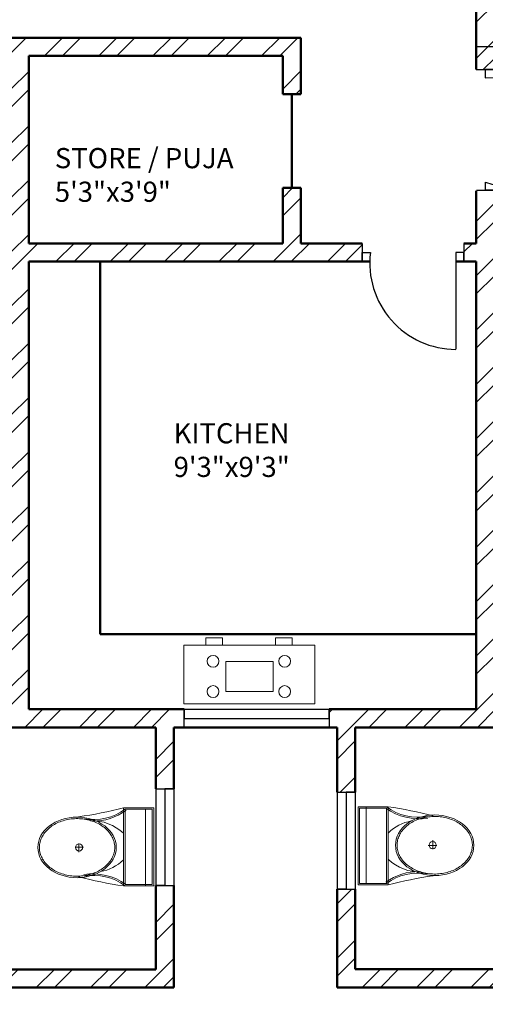
# Model space of a CAD drawing. Units: inches. Extents: x 963 to 2075, y 289 to 2657.
# Tile 4 of 98: x 1259 to 1374, y 1474 to 1718. Entities that reach past the tile are written whole.
import ezdxf

# ---------------------------------------------------------------- set-up
doc = ezdxf.new("R2010")
doc.units = ezdxf.units.IN
for name, color, linetype, lineweight in [('A-ANNO-DIMS', 2, 'Continuous', 18), ('A-AREA-IDEN', 7, 'Continuous', 18), ('A-DOOR', 4, 'Continuous', 25), ('A-FLOR-FIXT', 9, 'Continuous', 18), ('A-GLAZ', 3, 'Continuous', 25), ('A-WALL', 7, 'Continuous', 50), ('A-WALL-PATT', 8, 'Continuous', 13)]:
    doc.layers.add(name, color=color, linetype=linetype, lineweight=lineweight)
doc.styles.get("Standard").update_dxf_attribs({"font": 'arial.ttf'})
doc.dimstyles.get("Standard").update_dxf_attribs({"dimtxt": 0.18, "dimasz": 0.18, "dimexe": 0.18, "dimexo": 0.0625, "dimgap": 0.09, "dimtad": 0, "dimtih": 1, "dimtoh": 1, "dimdec": 4, "dimzin": 0, "dimdsep": 46, "dimtxsty": 'Standard', "dimcen": 0.09, "dimadec": 0, "dimazin": 0, "dimtfac": 1, "dimtdec": 4, "dimtofl": 0, "dimtmove": 0, "dimatfit": 3, "dimfxl": 1, "dimtolj": 1, "dimtzin": 0, "dimarcsym": 0})

# ---------------------------------------------------------------- blocks, each defined once
blk = doc.blocks.new('A$C31115884')
for p, q in [((283.1, 497.7), (223.4, 497.7)), ((257.5, 466.4), (257.5, 523.2)), ((0, 200), (0, 0)), ((520, 200), (0, 200)), ((520, 0), (520, 200)), ((10, 190), (10, 10)), ((510, 190), (10, 190)), ((510, 10), (510, 190)), ((510, 54.5), (0, 54.5)), ((10, 10), (510, 10)), ((0, 0), (520, 0))]:
    blk.add_line(p, q)
blk.add_circle((255.6, 496.4), 23.6)
for centre, radius, start, end in [((2777.7, -204.6), 2807, 165.4549, 171.71327), ((-294.5, 403.3), 364.7, 324.20913, 9.34987), ((-294.5, 403.3), 374.7, 324.20913, 9.34987), ((805.8, 403.3), 364.7, 170.65013, 215.79087), ((3237, 905), 2807, 188.28673, 194.5451), ((139.5, 406.2), 293.5, 315.84364, 2.65635), ((805.8, 403.3), 374.7, 179.20365, 215.79087), ((383.6, 406.2), 293.5, 190.27735, 224.15636)]:
    blk.add_arc(centre, radius, start, end)
blk.add_ellipse((256.2, 509.9), major_axis=(0, -260.7), ratio=0.772727)
blk.add_open_spline([(256.2, 259.2), (263.1, 259.2), (270, 259.7), (287.8, 262.3), (298.7, 265.1), (319.9, 273.1), (330.2, 278.4), (350.1, 291.1), (359.7, 298.7), (377.7, 315.9), (386.2, 325.5), (401.7, 346.6), (408.8, 358.1), (421.3, 382.5), (426.8, 395.5), (435.9, 422.4), (439.5, 436.4), (444.8, 465.1), (446.5, 479.7), (447.9, 509.2), (447.6, 524), (445, 553.3), (442.7, 567.8), (436.3, 596), (432.1, 609.7), (421.9, 636), (416, 648.6), (402.5, 672.1), (395, 683), (378.6, 703), (369.8, 712.1), (351.1, 728), (341.3, 734.8), (320.9, 746.2), (310.4, 750.7), (288.9, 757.3), (278, 759.4), (256, 761), (245, 760.6), (223.1, 757.2), (212.3, 754.3), (191.1, 746.1), (180.8, 740.7), (160.9, 727.8), (151.4, 720.1), (133.5, 702.7), (125.1, 693), (109.6, 671.7), (102.6, 660.2), (90.2, 635.7), (84.9, 622.7), (76, 595.6), (72.4, 581.6), (67.2, 552.9), (65.6, 538.2), (64.4, 508.8), (64.8, 494), (67.5, 464.7), (69.9, 450.2), (76.6, 422), (80.8, 408.3), (91.1, 382.2), (97.2, 369.7), (110.8, 346.3), (118.4, 335.4), (134.8, 315.6), (143.7, 306.7), (162.4, 290.9), (172.3, 284.2), (192.8, 273), (203.3, 268.6), (224.8, 262.2), (235.8, 260.2), (249.9, 259.3), (253, 259.2), (256.2, 259.2)], degree=3, knots=[0, 0, 0, 0, 0.110105, 0.110105, 0.285049, 0.285049, 0.459994, 0.459994, 0.634938, 0.634938, 0.809882, 0.809882, 0.984827, 0.984827, 1.159771, 1.159771, 1.334715, 1.334715, 1.50966, 1.50966, 1.684604, 1.684604, 1.859549, 1.859549, 2.034493, 2.034493, 2.209437, 2.209437, 2.384382, 2.384382, 2.559326, 2.559326, 2.73427, 2.73427, 2.909215, 2.909215, 3.084159, 3.084159, 3.259103, 3.259103, 3.434048, 3.434048, 3.608992, 3.608992, 3.783936, 3.783936, 3.958881, 3.958881, 4.133825, 4.133825, 4.30877, 4.30877, 4.483714, 4.483714, 4.658658, 4.658658, 4.833603, 4.833603, 5.008547, 5.008547, 5.183491, 5.183491, 5.358436, 5.358436, 5.53338, 5.53338, 5.708324, 5.708324, 5.883269, 5.883269, 6.058213, 6.058213, 6.233158, 6.233158, 6.283185, 6.283185, 6.283185, 6.283185])
blk = doc.blocks.new('DOOR-5')
for p, q in [((0, 38.25), (0, 33.75)), ((29.91, 38.25), (29.91, 33.75)), ((0, 33.75), (0, 36)), ((0, 36), (2, 36)), ((29.91, 36), (27.91, 36)), ((27.91, 36), (27.91, 0)), ((29.91, 33.75), (29.91, 36))]:
    blk.add_line(p, q)
blk.add_arc((27.91, 27.32), 27.32, 161.4794, 270)
blk = doc.blocks.new('*D38')
at = {"layer": 'A-ANNO-DIMS', "color": 0, "lineweight": -2, "transparency": 16777216}
for p, q in [((1371.88, 1705.97), (1371.87, 1711.82)), ((1372.05, 1711.64), (1389.86, 1711.69)), ((1409.94, 1711.73), (1392.12, 1711.69)), ((1410.13, 1706.06), (1410.12, 1711.92))]:
    blk.add_line(p, q, dxfattribs=at)
at = {"layer": 'A-ANNO-DIMS', "color": 0, "transparency": 16777216}
for points in [[(1372.05, 1711.67), (1372.05, 1711.61), (1371.87, 1711.64)], [(1409.94, 1711.76), (1409.94, 1711.7), (1410.12, 1711.74)]]:
    blk.add_solid(points, dxfattribs=at)
at = {"layer": 'Defpoints', "color": 0, "transparency": 16777216}
for p in [(1371.87, 1711.64), (1371.88, 1705.9), (1410.13, 1706)]:
    blk.add_point(p, dxfattribs=at)
at = {"layer": 'A-ANNO-DIMS', "color": 0, "transparency": 16777216, "insert": (1390.99, 1711.69), "char_height": 0.18, "attachment_point": 5}
blk.add_mtext('\\A1;DOOR D5 38 TYP.', dxfattribs=at)

msp = doc.modelspace()

# ---------------------------------------------------------------- hatches: boundary and pattern name
at = {"layer": 'A-WALL-PATT'}
h = msp.add_hatch(dxfattribs=at)
h.set_pattern_fill('ANSI32', color=256)
h.paths.add_polyline_path([(1296.92, 2558.32), (1203.92, 2558.32), (1203.92, 2493.82), (1191.53, 2493.82), (1191.53, 2489.32), (1211.06, 2489.32), (1211.06, 2492.02), (1211.06, 2493.82), (1208.42, 2493.82), (1208.42, 2553.82), (1292.42, 2553.82), (1292.42, 2538.86), (1296.92, 2538.86)])
h.paths.add_polyline_path([(1442.42, 2558.32), (1349.42, 2558.32), (1349.42, 2538.94), (1353.92, 2538.94), (1353.92, 2553.82), (1437.92, 2553.82), (1437.92, 2493.82), (1434.54, 2493.82), (1434.54, 2489.32), (1448.31, 2489.32), (1448.31, 2491.57), (1448.31, 2493.82), (1442.42, 2493.82)])
h.paths.add_polyline_path([(1415.55, 2491.57), (1415.55, 2493.82), (1340.94, 2493.82), (1340.94, 2489.32), (1371.92, 2489.32), (1371.92, 2378.32), (1367.6, 2378.32), (1367.6, 2373.82), (1371.92, 2373.82), (1371.92, 2355.19), (1376.42, 2355.19), (1376.42, 2489.32), (1415.55, 2489.32)])
h.paths.add_polyline_path([(1304.94, 2491.57), (1304.94, 2493.82), (1296.92, 2493.82), (1296.92, 2514.86), (1292.42, 2514.86), (1292.42, 2493.82), (1232.81, 2493.82), (1232.81, 2489.32), (1256.42, 2489.32), (1256.42, 2327.32), (1253.71, 2327.32), (1253.71, 2322.82), (1328.42, 2322.82), (1328.42, 2331.15), (1323.92, 2331.15), (1323.92, 2327.32), (1260.92, 2327.32), (1260.92, 2373.82), (1323.92, 2373.82), (1323.92, 2357.81), (1328.42, 2357.81), (1328.42, 2373.82), (1346.01, 2373.82), (1346.01, 2376.07), (1346.01, 2378.32), (1260.92, 2378.32), (1260.92, 2489.32), (1304.94, 2489.32)])
h.paths.add_polyline_path([(1226.65, 2327.32), (1124.42, 2327.32), (1124.42, 2347.45), (1119.92, 2347.45), (1119.92, 2322.82), (1163.42, 2322.82), (1163.42, 2305.43), (1165.67, 2305.43), (1167.92, 2305.43), (1167.92, 2322.82), (1226.65, 2322.82), (1226.65, 2325.07)])
h.paths.add_polyline_path([(1095.92, 2489.32), (1124.42, 2489.32), (1131.53, 2489.32), (1131.53, 2491.57), (1131.53, 2493.82), (1119.92, 2493.82), (1091.42, 2493.82), (1091.42, 2417.32), (1095.92, 2417.32), (1119.92, 2417.32), (1119.92, 2407.45), (1124.42, 2407.45), (1124.42, 2421.82), (1095.92, 2421.82)])
h.paths.add_polyline_path([(1512.92, 2558.32), (1508.42, 2558.32), (1508.42, 2493.82), (1503.4, 2493.82), (1503.4, 2489.32), (1508.42, 2489.32), (1508.42, 2327.32), (1376.42, 2327.32), (1376.42, 2330.27), (1371.92, 2330.27), (1371.92, 2298.74), (1376.42, 2298.74), (1376.42, 2322.82), (1508.42, 2322.82), (1508.42, 2165.32), (1504.26, 2165.32), (1504.26, 2160.82), (1508.42, 2160.82), (1508.42, 2108.32), (1512.92, 2108.32), (1512.92, 2160.82), (1516.18, 2160.82), (1516.18, 2163.07), (1516.18, 2165.32), (1512.92, 2165.32), (1512.92, 2322.82), (1644.92, 2322.82), (1644.92, 2298.74), (1649.42, 2298.74), (1649.42, 2322.82), (1649.42, 2330.94), (1647.17, 2330.94), (1644.92, 2330.94), (1644.92, 2327.32), (1512.92, 2327.32), (1512.92, 2489.32), (1516.76, 2489.32), (1516.76, 2491.57), (1516.76, 2493.82), (1512.92, 2493.82)])
h.paths.add_polyline_path([(1671.92, 2558.32), (1578.92, 2558.32), (1578.92, 2493.82), (1573.53, 2493.82), (1573.53, 2489.32), (1586.54, 2489.32), (1586.54, 2491.57), (1586.54, 2493.82), (1583.42, 2493.82), (1583.42, 2553.82), (1667.42, 2553.82), (1667.42, 2541.11), (1671.92, 2541.11)])
h.paths.add_polyline_path([(1681.26, 2493.82), (1671.92, 2493.82), (1671.92, 2517.11), (1667.42, 2517.11), (1667.42, 2493.82), (1610.22, 2493.82), (1610.22, 2489.32), (1644.92, 2489.32), (1644.92, 2357.87), (1649.42, 2357.87), (1649.42, 2373.82), (1652.2, 2373.82), (1652.2, 2375.83), (1652.2, 2378.32), (1649.42, 2378.32), (1649.42, 2489.32), (1681.26, 2489.32), (1681.26, 2491.57)])
h.paths.add_polyline_path([(1821.92, 2558.32), (1728.92, 2558.32), (1728.92, 2541), (1733.42, 2541), (1733.42, 2553.82), (1817.42, 2553.82), (1817.42, 2493.82), (1813.51, 2493.82), (1813.51, 2489.32), (1830.08, 2489.32), (1830.08, 2491.57), (1830.08, 2493.82), (1821.92, 2493.82)])
h.paths.add_polyline_path([(1794.24, 2493.82), (1717.26, 2493.82), (1717.26, 2489.32), (1760.42, 2489.32), (1760.42, 2378.32), (1674.4, 2378.32), (1674.4, 2373.82), (1692.92, 2373.82), (1692.92, 2356.95), (1697.42, 2356.95), (1697.42, 2373.82), (1760.42, 2373.82), (1760.42, 2327.32), (1697.42, 2327.32), (1697.42, 2333.34), (1692.92, 2333.34), (1692.92, 2322.82), (1768.04, 2322.82), (1768.04, 2325.07), (1768.04, 2327.32), (1764.92, 2327.32), (1764.92, 2489.32), (1794.24, 2489.32)])
h.paths.add_polyline_path([(1733.42, 2517), (1728.92, 2517), (1728.92, 2493.82), (1733.42, 2493.82)], flags=17)
h.paths.add_polyline_path([(1929.92, 2493.82), (1890.08, 2493.82), (1890.08, 2489.32), (1896.92, 2489.32), (1925.42, 2489.32), (1925.42, 2421.82), (1896.92, 2421.82), (1896.92, 2408.32), (1901.42, 2408.32), (1901.42, 2417.32), (1925.42, 2417.32), (1929.92, 2417.32)])
h.paths.add_polyline_path([(1901.42, 2348.32), (1896.92, 2348.32), (1896.92, 2327.32), (1800.42, 2327.32), (1800.42, 2322.82), (1853.42, 2322.82), (1853.42, 2309.45), (1857.92, 2309.45), (1857.92, 2322.82), (1901.42, 2322.82)])
h.paths.add_polyline_path([(1857.92, 2249.45), (1853.42, 2249.45), (1853.42, 2214.82), (1686.31, 2214.82), (1686.31, 2210.32), (1853.42, 2210.32), (1853.42, 2202.13), (1857.92, 2202.13), (1857.92, 2210.32)])
h.paths.add_polyline_path([(1857.92, 2142.13), (1853.42, 2142.13), (1853.42, 2115.42), (1841.42, 2115.42), (1841.42, 2088.53), (1841.42, 2046.95), (1845.92, 2046.95), (1845.92, 2110.92), (1905.92, 2110.92), (1905.92, 2092.52), (1910.42, 2092.52), (1910.42, 2115.42), (1857.92, 2115.42)])
h.paths.add_polyline_path([(1532.44, 1482.34), (1573.46, 1482.34), (1573.46, 1501), (1532.44, 1501)], flags=9)
h.paths.add_polyline_path([(1438.66, 1486.3), (1479.68, 1486.3), (1479.68, 1504.96), (1438.66, 1504.96)], flags=9)
h.paths.add_polyline_path([(1411.22, 1365.31), (1659.14, 1365.31), (1659.14, 1402.4), (1411.22, 1402.4)], flags=9)
h.paths.add_polyline_path([(1185.67, 2296.3), (1248.16, 2296.3), (1248.16, 2314.95), (1185.67, 2314.95)], flags=9)
h.paths.add_polyline_path([(1177.31, 2187.35), (1216.15, 2187.35), (1216.15, 2206.01), (1177.31, 2206.01)], flags=9)
h.paths.add_polyline_path([(1295.1, 1602.08), (1328.26, 1602.08), (1328.26, 1620.74), (1295.1, 1620.74)], flags=9)
h.paths.add_polyline_path([(1525.13, 2005.99), (1558.39, 2005.99), (1558.39, 2024.65), (1525.13, 2024.65)], flags=9)
h.paths.add_polyline_path([(1459.61, 1977.13), (1472.19, 1977.13), (1472.19, 1987.43), (1459.61, 1987.43)], flags=9)
h.paths.add_polyline_path([(1467.81, 2053.68), (1480.02, 2053.68), (1480.02, 2063.98), (1467.81, 2063.98)], flags=9)
h.paths.add_polyline_path([(1555.18, 2119.02), (1584.56, 2119.02), (1584.56, 2137.68), (1555.18, 2137.68)], flags=25)
h.paths.add_polyline_path([(1405.39, 2115.29), (1444.48, 2115.29), (1444.48, 2133.95), (1405.39, 2133.95)], flags=25)
h.paths.add_polyline_path([(1698.48, 2004.26), (1727.69, 2004.26), (1727.69, 2022.92), (1698.48, 2022.92)], flags=9)
h.paths.add_polyline_path([(1612.16, 1972.86), (1629.02, 1972.86), (1629.02, 1983.16), (1612.16, 1983.16)], flags=9)
h.paths.add_polyline_path([(1608.29, 2060.04), (1625.15, 2060.04), (1625.15, 2070.34), (1608.29, 2070.34)], flags=9)
h.paths.add_polyline_path([(1527.95, 1684.4), (1566.79, 1684.4), (1566.79, 1703.06), (1527.95, 1703.06)], flags=9)
h.paths.add_polyline_path([(1422.79, 1683.59), (1461.63, 1683.59), (1461.63, 1702.25), (1422.79, 1702.25)], flags=9)
h.paths.add_polyline_path([(1531.26, 1732.46), (1574.01, 1732.46), (1574.01, 1751.12), (1531.26, 1751.12)], flags=9)
h.paths.add_polyline_path([(1402.87, 1732.85), (1439.8, 1732.85), (1439.8, 1751.5), (1402.87, 1751.5)], flags=9)
h.paths.add_polyline_path([(1243.12, 1923.13), (1281.96, 1923.13), (1281.96, 1941.79), (1243.12, 1941.79)], flags=9)
h.paths.add_polyline_path([(1181.75, 1792.27), (1244.24, 1792.27), (1244.24, 1810.93), (1181.75, 1810.93)], flags=9)
h.paths.add_polyline_path([(1265.82, 1670.3), (1316.07, 1670.3), (1316.07, 1688.96), (1265.82, 1688.96)], flags=9)
h.paths.add_polyline_path([(1140.26, 1676.05), (1179.1, 1676.05), (1179.1, 1694.71), (1140.26, 1694.71)], flags=9)
h.paths.add_polyline_path([(1107.49, 1490.89), (1143.37, 1490.89), (1143.37, 1509.55), (1107.49, 1509.55)], flags=9)
h.paths.add_polyline_path([(1217.58, 1483.9), (1246.74, 1483.9), (1246.74, 1502.56), (1217.58, 1502.56)], flags=9)
h.paths.add_polyline_path([(1389.21, 1486.92), (1418.37, 1486.92), (1418.37, 1505.58), (1389.21, 1505.58)], flags=9)
h.paths.add_polyline_path([(1672.21, 1602.08), (1705.37, 1602.08), (1705.37, 1620.74), (1672.21, 1620.74)], flags=9)
h.paths.add_polyline_path([(1752.08, 1522.64), (1781.24, 1522.64), (1781.24, 1541.3), (1752.08, 1541.3)], flags=9)
h.paths.add_polyline_path([(1848.27, 1491.26), (1884.16, 1491.26), (1884.16, 1509.92), (1848.27, 1509.92)], flags=9)
h.paths.add_polyline_path([(1822.47, 1685.62), (1861.31, 1685.62), (1861.31, 1704.28), (1822.47, 1704.28)], flags=9)
h.paths.add_polyline_path([(1713.19, 1672.23), (1763.44, 1672.23), (1763.44, 1690.89), (1713.19, 1690.89)], flags=9)
h.paths.add_polyline_path([(1736.62, 1790.58), (1799.11, 1790.58), (1799.11, 1809.24), (1736.62, 1809.24)], flags=9)
h.paths.add_polyline_path([(1691.49, 1916.36), (1730.33, 1916.36), (1730.33, 1935.01), (1691.49, 1935.01)], flags=9)
h.paths.add_polyline_path([(1764.87, 1973.92), (1794.31, 1973.92), (1794.31, 1992.58), (1764.87, 1992.58)], flags=9)
h.paths.add_polyline_path([(1767.85, 2034.02), (1797.29, 2034.02), (1797.29, 2052.67), (1767.85, 2052.67)], flags=9)
h.paths.add_polyline_path([(1851.59, 2060.33), (1880.75, 2060.33), (1880.75, 2078.99), (1851.59, 2078.99)], flags=25)
h.paths.add_polyline_path([(1688.49, 2086.87), (1727.33, 2086.87), (1727.33, 2105.53), (1688.49, 2105.53)], flags=9)
h.paths.add_polyline_path([(1537.74, 2293.58), (1580.49, 2293.58), (1580.49, 2312.24), (1537.74, 2312.24)], flags=25)
h.paths.add_polyline_path([(1425.59, 2296.11), (1468.34, 2296.11), (1468.34, 2314.77), (1425.59, 2314.77)], flags=25)
h.paths.add_polyline_path([(1278.52, 2004.18), (1307.72, 2004.18), (1307.72, 2022.84), (1278.52, 2022.84)], flags=9)
h.paths.add_polyline_path([(1193.28, 1973.63), (1222.72, 1973.63), (1222.72, 1992.29), (1193.28, 1992.29)], flags=9)
h.paths.add_polyline_path([(1192.41, 2040.58), (1221.84, 2040.58), (1221.84, 2059.23), (1192.41, 2059.23)], flags=9)
h.paths.add_polyline_path([(1130.6, 1951.39), (1159.76, 1951.39), (1159.76, 1970.05), (1130.6, 1970.05)], flags=9)
h.paths.add_polyline_path([(1132.83, 2052.49), (1161.98, 2052.49), (1161.98, 2071.15), (1132.83, 2071.15)], flags=9)
h.paths.add_polyline_path([(1265.13, 2334.62), (1315.38, 2334.62), (1315.38, 2353.28), (1265.13, 2353.28)], flags=25)
h.paths.add_polyline_path([(1136.74, 2330.79), (1175.58, 2330.79), (1175.58, 2349.44), (1136.74, 2349.44)], flags=9)
h.paths.add_polyline_path([(1287.42, 2417.2), (1320.58, 2417.2), (1320.58, 2435.86), (1287.42, 2435.86)], flags=25)
h.paths.add_polyline_path([(1430.99, 2329.16), (1469.83, 2329.16), (1469.83, 2347.82), (1430.99, 2347.82)], flags=25)
h.paths.add_polyline_path([(1525.42, 2329.21), (1564.26, 2329.21), (1564.26, 2347.87), (1525.42, 2347.87)], flags=25)
h.paths.add_polyline_path([(1684.52, 2382.8), (1717.68, 2382.8), (1717.68, 2401.46), (1684.52, 2401.46)], flags=25)
h.paths.add_polyline_path([(1704.81, 2340.29), (1755.05, 2340.29), (1755.05, 2358.95), (1704.81, 2358.95)], flags=25)
h.paths.add_polyline_path([(1694.11, 2287.76), (1756.6, 2287.76), (1756.6, 2306.41), (1694.11, 2306.41)], flags=9)
h.paths.add_polyline_path([(1815.78, 2329.86), (1854.62, 2329.86), (1854.62, 2348.52), (1815.78, 2348.52)], flags=9)
h.paths.add_polyline_path([(1842.87, 2514.26), (1878.76, 2514.26), (1878.76, 2532.91), (1842.87, 2532.91)], flags=9)
h.paths.add_polyline_path([(1769.51, 2531.45), (1798.67, 2531.45), (1798.67, 2550.1), (1769.51, 2550.1)], flags=25)
h.paths.add_polyline_path([(1594.77, 2518.47), (1623.93, 2518.47), (1623.93, 2537.13), (1594.77, 2537.13)], flags=25)
h.paths.add_polyline_path([(1520.72, 2516.18), (1556.61, 2516.18), (1556.61, 2534.84), (1520.72, 2534.84)], flags=25)
h.paths.add_polyline_path([(1464.46, 2516.69), (1500.34, 2516.69), (1500.34, 2535.35), (1464.46, 2535.35)], flags=25)
h.paths.add_polyline_path([(1365.7, 2528.97), (1394.85, 2528.97), (1394.85, 2547.63), (1365.7, 2547.63)], flags=25)
h.paths.add_polyline_path([(1222.84, 2516.23), (1252, 2516.23), (1252, 2534.89), (1222.84, 2534.89)], flags=25)
h.paths.add_polyline_path([(1104.55, 2509.6), (1140.43, 2509.6), (1140.43, 2528.26), (1104.55, 2528.26)], flags=9)
h = msp.add_hatch(dxfattribs=at)
h.set_pattern_fill('ANSI32', color=256)
h.paths.add_polyline_path([(1335.97, 2212.57), (1335.97, 2214.82), (1167.92, 2214.82), (1167.92, 2245.43), (1163.42, 2245.43), (1163.42, 2210.32), (1163.42, 2194.81), (1167.92, 2194.81), (1167.92, 2210.32), (1335.97, 2210.32)])
h.paths.add_polyline_path([(1532.44, 1482.34), (1573.46, 1482.34), (1573.46, 1501), (1532.44, 1501)], flags=9)
h.paths.add_polyline_path([(1438.66, 1486.3), (1479.68, 1486.3), (1479.68, 1504.96), (1438.66, 1504.96)], flags=9)
h.paths.add_polyline_path([(1411.22, 1365.31), (1659.14, 1365.31), (1659.14, 1402.4), (1411.22, 1402.4)], flags=9)
h.paths.add_polyline_path([(1185.67, 2296.3), (1248.16, 2296.3), (1248.16, 2314.95), (1185.67, 2314.95)], flags=9)
h.paths.add_polyline_path([(1177.31, 2187.35), (1216.15, 2187.35), (1216.15, 2206.01), (1177.31, 2206.01)], flags=9)
h.paths.add_polyline_path([(1295.1, 1602.08), (1328.26, 1602.08), (1328.26, 1620.74), (1295.1, 1620.74)], flags=9)
h.paths.add_polyline_path([(1525.13, 2005.99), (1558.39, 2005.99), (1558.39, 2024.65), (1525.13, 2024.65)], flags=9)
h.paths.add_polyline_path([(1459.61, 1977.13), (1472.19, 1977.13), (1472.19, 1987.43), (1459.61, 1987.43)], flags=9)
h.paths.add_polyline_path([(1467.81, 2053.68), (1480.02, 2053.68), (1480.02, 2063.98), (1467.81, 2063.98)], flags=9)
h.paths.add_polyline_path([(1555.18, 2119.02), (1584.56, 2119.02), (1584.56, 2137.68), (1555.18, 2137.68)], flags=9)
h.paths.add_polyline_path([(1405.39, 2115.29), (1444.48, 2115.29), (1444.48, 2133.95), (1405.39, 2133.95)], flags=9)
h.paths.add_polyline_path([(1698.48, 2004.26), (1727.69, 2004.26), (1727.69, 2022.92), (1698.48, 2022.92)], flags=9)
h.paths.add_polyline_path([(1612.16, 1972.86), (1629.02, 1972.86), (1629.02, 1983.16), (1612.16, 1983.16)], flags=9)
h.paths.add_polyline_path([(1608.29, 2060.04), (1625.15, 2060.04), (1625.15, 2070.34), (1608.29, 2070.34)], flags=9)
h.paths.add_polyline_path([(1527.95, 1684.4), (1566.79, 1684.4), (1566.79, 1703.06), (1527.95, 1703.06)], flags=9)
h.paths.add_polyline_path([(1422.79, 1683.59), (1461.63, 1683.59), (1461.63, 1702.25), (1422.79, 1702.25)], flags=9)
h.paths.add_polyline_path([(1531.26, 1732.46), (1574.01, 1732.46), (1574.01, 1751.12), (1531.26, 1751.12)], flags=9)
h.paths.add_polyline_path([(1402.87, 1732.85), (1439.8, 1732.85), (1439.8, 1751.5), (1402.87, 1751.5)], flags=9)
h.paths.add_polyline_path([(1243.12, 1923.13), (1281.96, 1923.13), (1281.96, 1941.79), (1243.12, 1941.79)], flags=9)
h.paths.add_polyline_path([(1181.75, 1792.27), (1244.24, 1792.27), (1244.24, 1810.93), (1181.75, 1810.93)], flags=9)
h.paths.add_polyline_path([(1265.82, 1670.3), (1316.07, 1670.3), (1316.07, 1688.96), (1265.82, 1688.96)], flags=9)
h.paths.add_polyline_path([(1140.26, 1676.05), (1179.1, 1676.05), (1179.1, 1694.71), (1140.26, 1694.71)], flags=9)
h.paths.add_polyline_path([(1107.49, 1490.89), (1143.37, 1490.89), (1143.37, 1509.55), (1107.49, 1509.55)], flags=9)
h.paths.add_polyline_path([(1217.58, 1483.9), (1246.74, 1483.9), (1246.74, 1502.56), (1217.58, 1502.56)], flags=9)
h.paths.add_polyline_path([(1389.21, 1486.92), (1418.37, 1486.92), (1418.37, 1505.58), (1389.21, 1505.58)], flags=9)
h.paths.add_polyline_path([(1672.21, 1602.08), (1705.37, 1602.08), (1705.37, 1620.74), (1672.21, 1620.74)], flags=9)
h.paths.add_polyline_path([(1752.08, 1522.64), (1781.24, 1522.64), (1781.24, 1541.3), (1752.08, 1541.3)], flags=9)
h.paths.add_polyline_path([(1848.27, 1491.26), (1884.16, 1491.26), (1884.16, 1509.92), (1848.27, 1509.92)], flags=9)
h.paths.add_polyline_path([(1822.47, 1685.62), (1861.31, 1685.62), (1861.31, 1704.28), (1822.47, 1704.28)], flags=9)
h.paths.add_polyline_path([(1713.19, 1672.23), (1763.44, 1672.23), (1763.44, 1690.89), (1713.19, 1690.89)], flags=9)
h.paths.add_polyline_path([(1736.62, 1790.58), (1799.11, 1790.58), (1799.11, 1809.24), (1736.62, 1809.24)], flags=9)
h.paths.add_polyline_path([(1691.49, 1916.36), (1730.33, 1916.36), (1730.33, 1935.01), (1691.49, 1935.01)], flags=9)
h.paths.add_polyline_path([(1764.87, 1973.92), (1794.31, 1973.92), (1794.31, 1992.58), (1764.87, 1992.58)], flags=9)
h.paths.add_polyline_path([(1767.85, 2034.02), (1797.29, 2034.02), (1797.29, 2052.67), (1767.85, 2052.67)], flags=9)
h.paths.add_polyline_path([(1851.59, 2060.33), (1880.75, 2060.33), (1880.75, 2078.99), (1851.59, 2078.99)], flags=9)
h.paths.add_polyline_path([(1688.49, 2086.87), (1727.33, 2086.87), (1727.33, 2105.53), (1688.49, 2105.53)], flags=9)
h.paths.add_polyline_path([(1537.74, 2293.58), (1580.49, 2293.58), (1580.49, 2312.24), (1537.74, 2312.24)], flags=9)
h.paths.add_polyline_path([(1425.59, 2296.11), (1468.34, 2296.11), (1468.34, 2314.77), (1425.59, 2314.77)], flags=9)
h.paths.add_polyline_path([(1278.52, 2004.18), (1307.72, 2004.18), (1307.72, 2022.84), (1278.52, 2022.84)], flags=9)
h.paths.add_polyline_path([(1193.28, 1973.63), (1222.72, 1973.63), (1222.72, 1992.29), (1193.28, 1992.29)], flags=9)
h.paths.add_polyline_path([(1192.41, 2040.58), (1221.84, 2040.58), (1221.84, 2059.23), (1192.41, 2059.23)], flags=9)
h.paths.add_polyline_path([(1130.6, 1951.39), (1159.76, 1951.39), (1159.76, 1970.05), (1130.6, 1970.05)], flags=9)
h.paths.add_polyline_path([(1132.83, 2052.49), (1161.98, 2052.49), (1161.98, 2071.15), (1132.83, 2071.15)], flags=9)
h.paths.add_polyline_path([(1265.13, 2334.62), (1315.38, 2334.62), (1315.38, 2353.28), (1265.13, 2353.28)], flags=9)
h.paths.add_polyline_path([(1136.74, 2330.79), (1175.58, 2330.79), (1175.58, 2349.44), (1136.74, 2349.44)], flags=9)
h.paths.add_polyline_path([(1287.42, 2417.2), (1320.58, 2417.2), (1320.58, 2435.86), (1287.42, 2435.86)], flags=9)
h.paths.add_polyline_path([(1430.99, 2329.16), (1469.83, 2329.16), (1469.83, 2347.82), (1430.99, 2347.82)], flags=9)
h.paths.add_polyline_path([(1525.42, 2329.21), (1564.26, 2329.21), (1564.26, 2347.87), (1525.42, 2347.87)], flags=9)
h.paths.add_polyline_path([(1684.52, 2382.8), (1717.68, 2382.8), (1717.68, 2401.46), (1684.52, 2401.46)], flags=9)
h.paths.add_polyline_path([(1704.81, 2340.29), (1755.05, 2340.29), (1755.05, 2358.95), (1704.81, 2358.95)], flags=9)
h.paths.add_polyline_path([(1694.11, 2287.76), (1756.6, 2287.76), (1756.6, 2306.41), (1694.11, 2306.41)], flags=9)
h.paths.add_polyline_path([(1815.78, 2329.86), (1854.62, 2329.86), (1854.62, 2348.52), (1815.78, 2348.52)], flags=9)
h.paths.add_polyline_path([(1842.87, 2514.26), (1878.76, 2514.26), (1878.76, 2532.91), (1842.87, 2532.91)], flags=9)
h.paths.add_polyline_path([(1769.51, 2531.45), (1798.67, 2531.45), (1798.67, 2550.1), (1769.51, 2550.1)], flags=9)
h.paths.add_polyline_path([(1594.77, 2518.47), (1623.93, 2518.47), (1623.93, 2537.13), (1594.77, 2537.13)], flags=9)
h.paths.add_polyline_path([(1520.72, 2516.18), (1556.61, 2516.18), (1556.61, 2534.84), (1520.72, 2534.84)], flags=9)
h.paths.add_polyline_path([(1464.46, 2516.69), (1500.34, 2516.69), (1500.34, 2535.35), (1464.46, 2535.35)], flags=9)
h.paths.add_polyline_path([(1365.7, 2528.97), (1394.85, 2528.97), (1394.85, 2547.63), (1365.7, 2547.63)], flags=9)
h.paths.add_polyline_path([(1222.84, 2516.23), (1252, 2516.23), (1252, 2534.89), (1222.84, 2534.89)], flags=9)
h.paths.add_polyline_path([(1104.55, 2509.6), (1140.43, 2509.6), (1140.43, 2528.26), (1104.55, 2528.26)], flags=9)
h = msp.add_hatch(dxfattribs=at)
h.set_pattern_fill('ANSI32', color=256)
h.paths.add_polyline_path([(1473.61, 2163.07), (1473.61, 2165.32), (1376.42, 2165.32), (1376.42, 2227.98), (1371.92, 2227.98), (1371.92, 2214.82), (1368.41, 2214.82), (1368.41, 2210.32), (1371.92, 2210.32), (1371.92, 2160.82), (1395.92, 2160.82), (1395.92, 2090.32), (1217.34, 2090.32), (1217.34, 2085.82), (1395.92, 2085.82), (1458.92, 2085.82), (1458.92, 2108.32), (1454.42, 2108.32), (1454.42, 2090.32), (1400.42, 2090.32), (1400.42, 2160.82), (1473.61, 2160.82)])
h.paths.add_polyline_path([(1649.42, 2210.32), (1653.23, 2210.32), (1653.23, 2214.82), (1649.42, 2214.82), (1649.42, 2227.98), (1644.92, 2227.98), (1644.92, 2165.32), (1550.1, 2165.32), (1550.1, 2160.82), (1620.92, 2160.82), (1620.92, 2112.82), (1555.45, 2112.82), (1555.45, 2108.32), (1584.33, 2108.32), (1584.33, 2084.92), (1588.83, 2084.92), (1588.83, 2108.32), (1625.42, 2108.32), (1667.95, 2108.32), (1667.95, 2022.67), (1588.83, 2022.67), (1588.83, 2047.41), (1584.33, 2047.41), (1584.33, 1996), (1588.83, 1996), (1588.83, 2018.32), (1667.95, 2018.17), (1667.95, 1928.32), (1625.42, 1928.32), (1625.42, 1923.82), (1672.45, 1923.82), (1672.45, 1928.32), (1672.45, 1946.66), (1785.45, 1946.66), (1785.45, 1951.16), (1743.03, 1951.16), (1743.03, 2017.92), (1841.42, 2017.92), (1841.42, 2014.77), (1845.92, 2014.77), (1845.92, 2017.92), (1905.92, 2017.92), (1905.92, 1987.51), (1910.42, 1987.51), (1910.42, 2022.42), (1910.42, 2068.52), (1905.92, 2068.52), (1905.92, 2022.42), (1845.92, 2022.42), (1845.92, 2025.85), (1843.67, 2025.85), (1841.42, 2025.85), (1841.42, 2022.42), (1743.03, 2022.42), (1743.03, 2084.03), (1768.45, 2084.03), (1785.45, 2084.03), (1785.45, 2088.53), (1672.45, 2088.53), (1672.45, 2112.82), (1667.95, 2112.82), (1625.42, 2112.82), (1625.42, 2160.82), (1649.42, 2160.82)])
h.paths.add_polyline_path([(1672.45, 2084.03), (1738.53, 2084.03), (1738.53, 1951.16), (1672.45, 1951.16)], flags=16)
h.paths.add_polyline_path([(1672.45, 2084.03), (1738.53, 2084.03), (1705.49, 2017.6)], flags=0)
h.paths.add_polyline_path([(1262.77, 2085.82), (1258.27, 2085.82), (1258.27, 2023.28), (1184.42, 2023.28), (1184.42, 2018.78), (1258.27, 2018.78), (1258.27, 1950.82), (1262.77, 1950.82)])
h.paths.add_polyline_path([(1312.27, 2085.82), (1307.77, 2085.82), (1307.77, 1950.82), (1312.27, 1950.82)])
h.paths.add_polyline_path([(1458.92, 1950.82), (1395.92, 1950.82), (1216.57, 1950.82), (1216.57, 1946.32), (1346.42, 1946.32), (1395.92, 1946.32), (1395.92, 1875.82), (1371.92, 1875.82), (1371.92, 1826.32), (1368.93, 1826.32), (1368.93, 1821.82), (1371.92, 1821.82), (1371.92, 1813.62), (1376.42, 1813.62), (1376.42, 1871.32), (1474.5, 1871.32), (1474.5, 1873.57), (1474.5, 1875.82), (1400.42, 1875.82), (1400.42, 1946.32), (1454.42, 1946.32), (1454.42, 1928.32), (1458.92, 1928.32)])
h.paths.add_polyline_path([(1184.42, 2120.78), (1167.92, 2120.78), (1167.92, 2134.81), (1165.67, 2134.81), (1163.42, 2134.81), (1163.42, 2120.78), (1119.92, 2120.78), (1119.92, 2098.1), (1124.42, 2098.1), (1124.42, 2116.28), (1167.92, 2116.28), (1179.92, 2116.28), (1179.92, 2045.92), (1184.42, 2045.92), (1184.42, 2090.32), (1184.42, 2116.28)])
h.paths.add_polyline_path([(1124.42, 2018.78), (1179.92, 2018.78), (1179.92, 2016.29), (1184.42, 2016.29), (1184.42, 2023.28), (1184.42, 2026.59), (1182.17, 2026.59), (1179.92, 2026.59), (1179.92, 2023.28), (1124.42, 2023.28), (1124.42, 2074.1), (1119.92, 2074.1), (1119.92, 2018.78), (1119.92, 1979.63), (1124.42, 1979.63)])
h.paths.add_polyline_path([(1184.42, 1925.78), (1184.42, 1946.32), (1184.42, 1996.07), (1182.17, 1996.07), (1179.92, 1996.07), (1179.92, 1925.78), (1124.42, 1925.78), (1124.42, 1955.63), (1119.92, 1955.5), (1119.92, 1921.28), (1158.92, 1921.28), (1158.92, 1909.98), (1163.42, 1909.98), (1163.42, 1921.28), (1184.42, 1921.28)])
h.paths.add_polyline_path([(1341.45, 1826.32), (1163.42, 1826.32), (1163.42, 1849.98), (1158.92, 1849.98), (1158.92, 1821.82), (1158.92, 1804.03), (1163.42, 1804.03), (1163.42, 1821.82), (1341.45, 1821.82)])
h.paths.add_polyline_path([(1222.98, 1713.82), (1163.42, 1713.82), (1163.42, 1744.03), (1161.17, 1744.03), (1158.92, 1744.03), (1158.92, 1713.82), (1119.92, 1713.82), (1119.92, 1694.65), (1124.42, 1694.65), (1124.42, 1709.32), (1158.92, 1709.32), (1222.98, 1709.32)])
h.paths.add_polyline_path([(1328.42, 1713.82), (1252.04, 1713.82), (1252.04, 1711.57), (1252.04, 1709.32), (1256.42, 1709.32), (1256.42, 1547.32), (1232.94, 1547.32), (1232.94, 1545.07), (1232.94, 1542.82), (1292.42, 1542.82), (1292.42, 1527.63), (1296.92, 1527.63), (1296.92, 1542.82), (1299.46, 1542.82), (1299.46, 1547.32), (1260.92, 1547.32), (1260.92, 1658.32), (1343.66, 1658.32), (1343.66, 1660.57), (1343.66, 1662.82), (1328.42, 1662.82), (1328.42, 1676.59), (1327.4, 1676.59), (1323.92, 1676.59), (1323.92, 1662.82), (1260.92, 1662.82), (1260.92, 1709.32), (1323.92, 1709.32), (1323.92, 1699.85), (1328.42, 1699.85)])
h.paths.add_polyline_path([(1649.42, 1875.82), (1625.42, 1875.82), (1625.42, 1928.32), (1620.92, 1928.32), (1588.83, 1928.32), (1588.83, 1950.59), (1584.33, 1950.59), (1584.33, 1928.32), (1555.45, 1928.32), (1555.45, 1923.82), (1620.92, 1923.82), (1620.92, 1875.82), (1548.95, 1875.82), (1548.95, 1873.57), (1548.95, 1871.32), (1644.92, 1871.32), (1644.92, 1813.62), (1649.42, 1813.62), (1649.42, 1821.82), (1652.04, 1821.82), (1652.04, 1824.07), (1652.04, 1826.32), (1649.42, 1826.32)])
h.paths.add_polyline_path([(1512.92, 1871.32), (1516.48, 1871.32), (1516.48, 1875.82), (1512.92, 1875.82), (1512.92, 1923.82), (1512.92, 1928.32), (1512.92, 1930.83), (1508.42, 1930.83), (1508.42, 1875.82), (1504.41, 1875.82), (1504.41, 1871.32), (1508.42, 1871.32), (1508.42, 1713.82), (1376.42, 1713.82), (1376.42, 1743.32), (1371.92, 1743.32), (1371.92, 1709.32), (1371.92, 1706.01), (1376.42, 1706.01), (1376.42, 1709.32), (1508.42, 1709.32), (1508.42, 1547.32), (1501.87, 1547.32), (1501.87, 1542.82), (1508.42, 1542.82), (1508.42, 1482.82), (1508.42, 1436.32), (1512.92, 1436.32), (1512.92, 1542.82), (1519.32, 1542.82), (1519.32, 1545.07), (1519.32, 1547.32), (1512.92, 1547.32), (1512.92, 1709.32), (1644.92, 1709.32), (1644.92, 1707.55), (1649.42, 1707.55), (1649.42, 1709.32), (1649.42, 1743.32), (1644.92, 1743.32), (1644.92, 1713.82), (1512.92, 1713.82)])
h.paths.add_polyline_path([(1129.88, 1545.07), (1129.88, 1547.32), (1124.42, 1547.32), (1095.92, 1547.32), (1095.92, 1614.82), (1124.42, 1614.82), (1124.42, 1619.32), (1095.92, 1619.32), (1091.42, 1619.32), (1091.42, 1542.82), (1095.92, 1542.82), (1119.92, 1542.82), (1129.88, 1542.82)])
h.paths.add_polyline_path([(1208.42, 1542.82), (1211.74, 1542.82), (1211.74, 1547.32), (1198.85, 1547.32), (1198.85, 1542.82), (1203.92, 1542.82), (1203.92, 1478.32), (1208.42, 1478.32), (1296.92, 1478.32), (1296.92, 1503.63), (1292.42, 1503.63), (1292.42, 1482.82), (1208.42, 1482.82)])
h.paths.add_polyline_path([(1430.42, 1542.82), (1435.7, 1542.82), (1435.7, 1545.07), (1435.7, 1547.32), (1422.66, 1547.32), (1422.66, 1545.07), (1422.66, 1542.82), (1425.92, 1542.82), (1425.92, 1482.86), (1341.92, 1482.86), (1341.92, 1502.73), (1337.42, 1502.73), (1337.42, 1478.36), (1425.92, 1478.36), (1425.92, 1440.82), (1425.92, 1436.32), (1430.42, 1436.32)])
h.paths.add_polyline_path([(1698.48, 2004.26), (1727.69, 2004.26), (1727.69, 2022.92), (1698.48, 2022.92)], flags=8)
h = msp.add_hatch(dxfattribs=at)
h.set_pattern_fill('ANSI32', color=256)
h.paths.add_polyline_path([(1910.42, 1929.42), (1910.42, 1963.51), (1905.92, 1963.51), (1905.92, 1929.42), (1845.92, 1929.42), (1845.92, 1993.37), (1843.67, 1993.37), (1841.42, 1993.37), (1841.42, 1951.16), (1841.42, 1924.92), (1853.42, 1924.92), (1853.42, 1913.07), (1857.92, 1913.07), (1857.92, 1924.92), (1910.42, 1924.92)])
h.paths.add_polyline_path([(1857.92, 1853.07), (1853.42, 1853.07), (1853.42, 1826.32), (1841.42, 1826.32), (1674.48, 1826.32), (1674.48, 1821.82), (1853.42, 1821.82), (1857.92, 1821.82)])
h.paths.add_polyline_path([(1857.92, 1821.82), (1853.42, 1821.82), (1853.42, 1807.79), (1857.92, 1807.79)])
h.paths.add_polyline_path([(1857.92, 1747.79), (1853.42, 1747.79), (1853.42, 1713.82), (1809.34, 1713.82), (1809.34, 1709.32), (1905.92, 1709.32), (1905.92, 1688.32), (1910.42, 1688.32), (1910.42, 1713.82), (1857.92, 1713.82)])
h.paths.add_polyline_path([(1830.92, 1542.82), (1837.43, 1542.82), (1837.43, 1545.07), (1837.43, 1547.32), (1823.42, 1547.32), (1823.42, 1545.07), (1823.42, 1542.82), (1826.42, 1542.82), (1826.42, 1482.82), (1742.42, 1482.82), (1742.42, 1505.39), (1737.92, 1505.39), (1737.92, 1478.32), (1830.92, 1478.32)])
h.paths.add_polyline_path([(1938.92, 1619.32), (1934.42, 1619.32), (1910.42, 1619.32), (1910.42, 1628.32), (1908.17, 1628.32), (1905.92, 1628.32), (1905.92, 1614.82), (1934.42, 1614.82), (1934.42, 1547.32), (1905.92, 1547.32), (1899.59, 1547.32), (1899.59, 1542.82), (1910.42, 1542.82), (1938.92, 1542.82)])
h.paths.add_polyline_path([(1803.68, 1547.32), (1773.92, 1547.32), (1773.92, 1709.32), (1777.76, 1709.32), (1777.76, 1713.82), (1701.92, 1713.82), (1701.92, 1697.8), (1706.42, 1697.8), (1706.42, 1709.32), (1769.42, 1709.32), (1769.42, 1662.82), (1706.42, 1662.82), (1706.42, 1674.38), (1701.92, 1674.38), (1701.92, 1662.82), (1675.67, 1662.82), (1675.67, 1658.32), (1769.42, 1658.32), (1769.42, 1547.32), (1729.17, 1547.32), (1729.17, 1542.82), (1737.92, 1542.82), (1737.92, 1529.39), (1742.42, 1529.39), (1742.42, 1542.82), (1803.68, 1542.82)])
h.paths.add_polyline_path([(1595.42, 1542.82), (1599.24, 1542.82), (1599.24, 1547.32), (1584.36, 1547.32), (1584.36, 1542.82), (1590.92, 1542.82), (1590.92, 1436.32), (1595.42, 1436.32), (1595.42, 1440.82)])
h.paths.add_polyline_path([(1693.17, 1547.32), (1649.42, 1547.32), (1649.42, 1658.32), (1652.1, 1658.32), (1652.1, 1660.57), (1652.1, 1662.82), (1649.42, 1662.82), (1649.42, 1680.94), (1647.17, 1680.94), (1644.92, 1680.94), (1644.92, 1547.32), (1622.42, 1547.32), (1622.42, 1545.07), (1622.42, 1542.82), (1649.42, 1542.82), (1679.42, 1542.82), (1679.42, 1529.85), (1681.67, 1529.85), (1683.92, 1529.85), (1683.92, 1542.82), (1693.17, 1542.82), (1693.17, 1545.07)])
h.paths.add_polyline_path([(1683.92, 1505.85), (1679.42, 1505.85), (1679.42, 1483.8), (1595.42, 1483.8), (1595.42, 1479.3), (1683.92, 1479.3)])
h.paths.add_polyline_path([(1402.99, 1547.32), (1376.42, 1547.32), (1376.42, 1675.89), (1374.17, 1675.89), (1371.92, 1675.89), (1371.92, 1662.82), (1368.88, 1662.82), (1368.88, 1658.32), (1371.92, 1658.32), (1371.92, 1547.32), (1335.46, 1547.32), (1335.46, 1542.82), (1337.42, 1542.82), (1337.42, 1526.73), (1341.92, 1526.73), (1341.92, 1542.82), (1371.92, 1542.82), (1402.99, 1542.82)])

# ---------------------------------------------------------------- linework, layer by layer
at = {"layer": 'A-DOOR'}
for p, q in [((1343.66, 1662.82), (1343.66, 1658.32)), ((1368.88, 1662.82), (1368.88, 1658.32)), ((1343.66, 1658.32), (1343.66, 1660.57)), ((1343.66, 1660.57), (1345.66, 1660.57)), ((1368.88, 1660.57), (1366.88, 1660.57)), ((1366.88, 1660.57), (1366.88, 1636.57)), ((1368.88, 1658.32), (1368.88, 1660.57))]:
    msp.add_line(p, q, dxfattribs=at)
msp.add_arc((1366.88, 1657.94), 21.38, 172.9505, 270, dxfattribs=at)
at = {"layer": 'A-FLOR-FIXT'}
for points in [[(1304.87, 1563.23), (1309.02, 1563.23), (1309.02, 1565.05), (1304.87, 1565.05)], [(1322.1, 1563.23), (1326.25, 1563.23), (1326.25, 1565.05), (1322.1, 1565.05)], [(1299.36, 1563.23), (1331.92, 1563.23), (1331.92, 1548.63), (1299.36, 1548.63)], [(1309.8, 1559.17), (1321.54, 1559.17), (1321.54, 1551.69), (1309.8, 1551.69)]]:
    msp.add_lwpolyline(points, close=True, dxfattribs=at)
for centre in [(1306.63, 1559.21), (1324.4, 1559.21), (1306.63, 1551.69), (1324.4, 1551.69)]:
    msp.add_circle(centre, 1.48, dxfattribs=at)
at = {"layer": 'A-GLAZ'}
for p, q in [((1299.46, 1542.82), (1299.46, 1547.32)), ((1299.46, 1547.32), (1299.46, 1545.07)), ((1299.46, 1547.32), (1335.46, 1547.32)), ((1335.46, 1545.07), (1335.46, 1547.32)), ((1335.46, 1547.32), (1335.46, 1542.82)), ((1299.46, 1545.07), (1335.46, 1545.07)), ((1335.46, 1542.82), (1299.46, 1542.82)), ((1299.46, 1542.82), (1299.46, 1542.82)), ((1292.42, 1527.63), (1296.92, 1527.63)), ((1292.42, 1527.63), (1292.42, 1503.63)), ((1296.92, 1527.63), (1294.67, 1527.63)), ((1294.67, 1527.63), (1294.67, 1503.63)), ((1296.92, 1527.63), (1296.92, 1503.63)), ((1337.42, 1526.73), (1341.92, 1526.73)), ((1337.42, 1526.73), (1337.42, 1502.73)), ((1341.92, 1526.73), (1339.67, 1526.73)), ((1339.67, 1526.73), (1339.67, 1502.73)), ((1341.92, 1526.73), (1341.92, 1502.73)), ((1294.67, 1503.63), (1292.42, 1503.63)), ((1292.42, 1503.63), (1296.92, 1503.63)), ((1339.67, 1502.73), (1337.42, 1502.73)), ((1337.42, 1502.73), (1341.92, 1502.73))]:
    msp.add_line(p, q, dxfattribs=at)
at = {"layer": 'A-WALL'}
for p, q in [((1371.92, 1743.32), (1371.92, 1709.32)), ((1252.04, 1713.82), (1328.42, 1713.82)), ((1328.42, 1713.82), (1328.42, 1699.85)), ((1323.92, 1709.32), (1260.92, 1709.32)), ((1260.92, 1709.32), (1260.92, 1662.82)), ((1323.92, 1709.32), (1323.92, 1699.85)), ((1371.92, 1709.32), (1371.92, 1706.01)), ((1323.92, 1699.85), (1328.42, 1699.85)), ((1326.17, 1699.85), (1326.17, 1676.59)), ((1323.92, 1676.59), (1327.4, 1676.59)), ((1323.92, 1676.59), (1323.92, 1662.82)), ((1327.4, 1676.59), (1328.42, 1676.59)), ((1328.42, 1676.59), (1328.42, 1662.82)), ((1371.92, 1675.89), (1371.92, 1662.82)), ((1260.92, 1662.82), (1323.92, 1662.82)), ((1328.42, 1662.82), (1343.66, 1662.82)), ((1368.88, 1662.82), (1371.92, 1662.82)), ((1260.92, 1658.32), (1345.5, 1658.32)), ((1260.92, 1658.32), (1260.92, 1547.32)), ((1278.62, 1658.32), (1278.62, 1565.9)), ((1366.88, 1658.32), (1371.92, 1658.32)), ((1371.92, 1658.32), (1371.92, 1547.32)), ((1278.62, 1565.9), (1371.92, 1565.9)), ((1260.92, 1547.32), (1299.46, 1547.32)), ((1335.46, 1547.32), (1371.92, 1547.32)), ((1292.42, 1542.82), (1232.42, 1542.82)), ((1292.42, 1542.82), (1292.42, 1527.63)), ((1296.92, 1542.82), (1296.92, 1527.63)), ((1337.42, 1542.82), (1296.92, 1542.82)), ((1337.42, 1542.82), (1337.42, 1526.73)), ((1371.92, 1542.82), (1341.92, 1542.82)), ((1341.92, 1542.82), (1341.92, 1526.73)), ((1404.46, 1542.82), (1371.92, 1542.82)), ((1292.42, 1503.63), (1292.42, 1482.82)), ((1296.92, 1503.63), (1296.92, 1478.32)), ((1337.42, 1502.73), (1337.42, 1478.36)), ((1341.92, 1502.73), (1341.92, 1482.86)), ((1208.42, 1482.82), (1292.42, 1482.82)), ((1341.92, 1482.86), (1425.92, 1482.86)), ((1296.92, 1478.32), (1208.42, 1478.32)), ((1425.92, 1478.36), (1337.42, 1478.36))]:
    msp.add_line(p, q, dxfattribs=at)

# ---------------------------------------------------------------- block references
at = {"layer": 'A-DOOR', "rotation": 90.14142652708767}
msp.add_blockref('DOOR-5', (1410.2, 1676.09), dxfattribs=at)
at = {"layer": 'A-FLOR-FIXT', "xscale": 0.0372717239612423, "yscale": 0.0372717239612423, "zscale": 0.0372717239612423}
for p, rotation in [((1291.91, 1503.52), 89.99999999999999), ((1342.61, 1523.15), 270)]:
    msp.add_blockref('A$C31115884', p, dxfattribs=dict(at, rotation=rotation))

# ---------------------------------------------------------------- texts
at = {"layer": 'A-AREA-IDEN', "char_height": 5, "attachment_point": 1}
for s, width, insert in [('STORE / PUJA\\P5\'3"x3\'9"', 92.7566, (1267.39, 1686.47)), ('KITCHEN\\P9\'3"x9\'3"', 120.9099, (1296.86, 1618.25))]:
    msp.add_mtext_dynamic_manual_height_columns(s, width=width, gutter_width=12.5, heights=[0], dxfattribs=dict(at, insert=insert))

# ---------------------------------------------------------------- dimensions: what is measured, and where the dimension line sits
at = {"layer": 'A-ANNO-DIMS'}
dim = msp.add_linear_dim(base=(1371.87, 1711.64), p1=(1410.13, 1706), p2=(1371.88, 1705.9), angle=180.1414, text='DOOR D5 <> TYP.', dimstyle='Standard', override={"dimdec": 0, "dimlfac": 1, "dimrnd": 0, "dimzin": 0, "dimdsep": 46, "dimlunit": 2}, dxfattribs=at)
dim.commit()
dim.dimension.update_dxf_attribs({"geometry": '*D38', "text_midpoint": (1390.99, 1711.69)})

doc.saveas('drawing.dxf')
